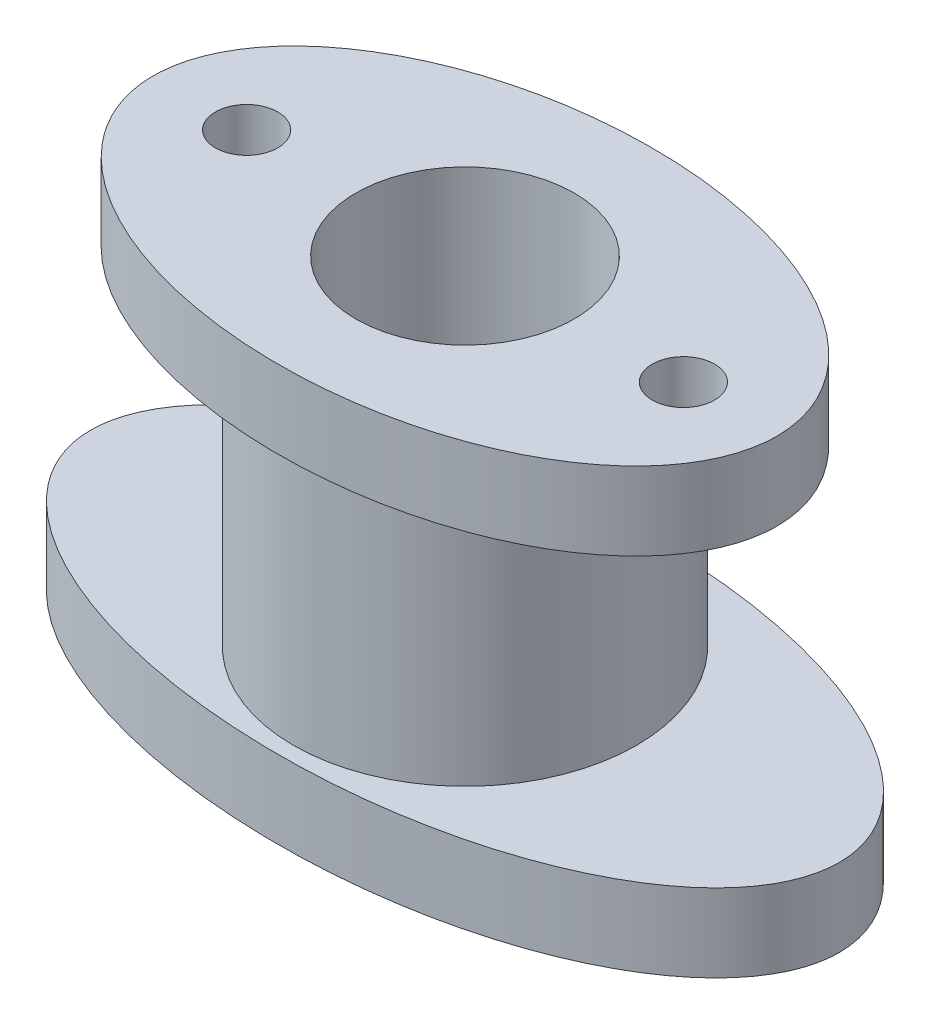
SolidWorks part; units mm, degrees
material "Plain Carbon Steel"
ref_plane "Front Plane" through (0, 0, 0) normal (0, 0, 1) x (1, 0, 0)
ref_plane "Top Plane" through (0, 0, 0) normal (0, 1, 0) x (1, 0, 0)
ref_plane "Right Plane" through (0, 0, 0) normal (1, 0, 0) x (0, 0, -1)
sketch "Base Flange Sketch" plane through (0, 0, 0) normal (0, 1, 0) x (1, 0, 0)
  ellipse E0 centre (0, 0) end of major axis (72, 0) minor radius 36
  dimension "D1" = 36
  dimension "D2" = 144
extrude "Base Flange" add sketch "Base Flange Sketch" along normal blind 15
sketch "Center Boss Sketch" plane through (0, 15, 0) normal (0, 1, 0) x (1, 0, 0)
  circle A0 centre (0, 0) radius 33
  dimension "D1" = 66
extrude "Center Boss Ø66" add sketch "Center Boss Sketch" along normal blind 50
sketch "Top Flange Sketch" plane through (0, 65, 0) normal (0, 1, 0) x (1, 0, 0)
  circle A0 centre (-42, 0) radius 6
  circle A1 centre (42, 0) radius 6
  ellipse E0 centre (0, 0) end of major axis (60, 0) minor radius 36
  dimension "D3" = 84
  dimension "D5" = 12
  dimension "D6" = 12
  dimension "D1" = 36
  dimension "D2" = 120
  dimension "D4" = 42
extrude "Top Flange with Holes 2xØ12" add sketch "Top Flange Sketch" along normal blind 15
sketch "Bore Sketch" plane through (0, 80, 0) normal (0, 1, 0) x (1, 0, 0)
  circle A0 centre (0, 0) radius 21
  dimension "D1" = 42
extrude "Bore Ø42" cut sketch "Bore Sketch" against normal blind 65
